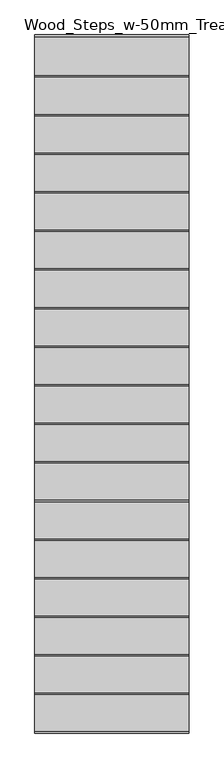
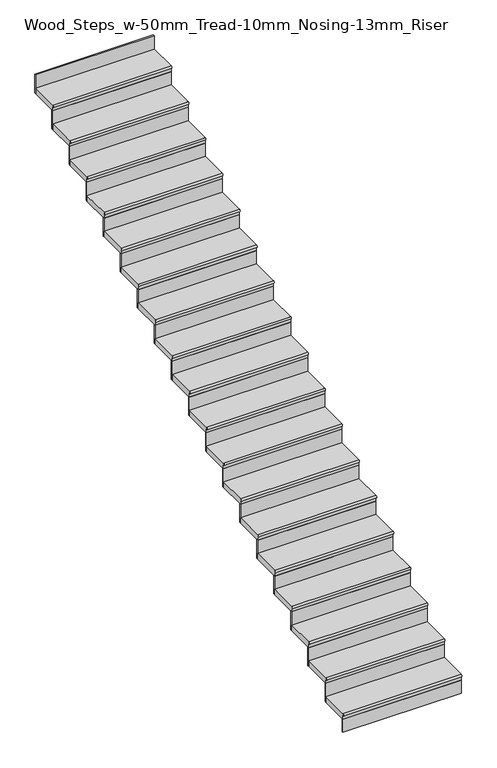
"""IFC4 building model written with IfcOpenShell, lengths in millimetres: stair flight geometry, Wood_Steps_w-50mm_Tread-10mm_Nosing-13mm_Riser."""

from ifc_helpers import new_model, si_unit, point, frame, frame_2d, origin, origin_with_axes, place, context, project, spatial, polyline, circle_curve, trimmed, segment, composite_curve, outline, extrude, source, transform, mapped, element, save


def wood_steps_w_50mm_tread_10mm_nosing_13mm_riser_22d6e456(model_context):
    return source(origin(), model_context, "Body", "SweptSolid", [
        extrude(outline(composite_curve([segment(polyline([(10202.4990528, 168.4210526), (10452.4990528, 168.4210526), (10452.4990528, 118.4210526), (10202.4990528, 118.4210526), (10202.4990528, 148.4210526)]), True, "CONTINUOUS"), segment(trimmed(circle_curve(frame_2d((10202.4990528, 158.4210526)), 10.0), [point((10202.4990528, 148.4210526))], [point((10202.4990528, 168.4210526))], False, "CARTESIAN"), True, "CONTINUOUS")], self_intersect=False)), frame((-6660.2000057, 0.0, 0.0), z_axis=(1.0, 0.0, 0.0), x_axis=(0.0, 1.0, 0.0)), (0.0, 0.0, 1.0), 1000.0),
        extrude(outline(polyline([(-5660.2000057, 10214.9990528), (-5660.2000057, 10202.4990528), (-6660.2000057, 10202.4990528), (-6660.2000057, 10214.9990528), (-5660.2000057, 10214.9990528)])), origin_with_axes(), (0.0, 0.0, 1.0), 118.4210526),
        extrude(outline(polyline([(-5660.2000057, 10464.9990528), (-5660.2000057, 10452.4990528), (-6660.2000057, 10452.4990528), (-6660.2000057, 10464.9990528), (-5660.2000057, 10464.9990528)])), frame((0.0, 0.0, 118.4210526), z_axis=(0.0, 0.0, 1.0), x_axis=(1.0, 0.0, 0.0)), (0.0, 0.0, 1.0), 168.4210526),
        extrude(outline(composite_curve([segment(polyline([(10452.4990528, 336.8421053), (10702.4990528, 336.8421053), (10702.4990528, 286.8421053), (10452.4990528, 286.8421053), (10452.4990528, 316.8421053)]), True, "CONTINUOUS"), segment(trimmed(circle_curve(frame_2d((10452.4990528, 326.8421053)), 10.0), [point((10452.4990528, 316.8421053))], [point((10452.4990528, 336.8421053))], False, "CARTESIAN"), True, "CONTINUOUS")], self_intersect=False)), frame((-6660.2000057, 0.0, 0.0), z_axis=(1.0, 0.0, 0.0), x_axis=(0.0, 1.0, 0.0)), (0.0, 0.0, 1.0), 1000.0),
        extrude(outline(polyline([(-5660.2000057, 10714.9990528), (-5660.2000057, 10702.4990528), (-6660.2000057, 10702.4990528), (-6660.2000057, 10714.9990528), (-5660.2000057, 10714.9990528)])), frame((0.0, 0.0, 286.8421053), z_axis=(0.0, 0.0, 1.0), x_axis=(1.0, 0.0, 0.0)), (0.0, 0.0, 1.0), 168.4210526),
        extrude(outline(composite_curve([segment(polyline([(10702.4990528, 505.2631579), (10952.4990528, 505.2631579), (10952.4990528, 455.2631579), (10702.4990528, 455.2631579), (10702.4990528, 485.2631579)]), True, "CONTINUOUS"), segment(trimmed(circle_curve(frame_2d((10702.4990528, 495.2631579)), 10.0), [point((10702.4990528, 485.2631579))], [point((10702.4990528, 505.2631579))], False, "CARTESIAN"), True, "CONTINUOUS")], self_intersect=False)), frame((-6660.2000057, 0.0, 0.0), z_axis=(1.0, 0.0, 0.0), x_axis=(0.0, 1.0, 0.0)), (0.0, 0.0, 1.0), 1000.0),
        extrude(outline(polyline([(-5660.2000057, 10964.9990528), (-5660.2000057, 10952.4990528), (-6660.2000057, 10952.4990528), (-6660.2000057, 10964.9990528), (-5660.2000057, 10964.9990528)])), frame((0.0, 0.0, 455.2631579), z_axis=(0.0, 0.0, 1.0), x_axis=(1.0, 0.0, 0.0)), (0.0, 0.0, 1.0), 168.4210526),
        extrude(outline(composite_curve([segment(polyline([(10952.4990528, 673.6842105), (11202.4990528, 673.6842105), (11202.4990528, 623.6842105), (10952.4990528, 623.6842105), (10952.4990528, 653.6842105)]), True, "CONTINUOUS"), segment(trimmed(circle_curve(frame_2d((10952.4990528, 663.6842105)), 10.0), [point((10952.4990528, 653.6842105))], [point((10952.4990528, 673.6842105))], False, "CARTESIAN"), True, "CONTINUOUS")], self_intersect=False)), frame((-6660.2000057, 0.0, 0.0), z_axis=(1.0, 0.0, 0.0), x_axis=(0.0, 1.0, 0.0)), (0.0, 0.0, 1.0), 1000.0),
        extrude(outline(polyline([(-5660.2000057, 11214.9990528), (-5660.2000057, 11202.4990528), (-6660.2000057, 11202.4990528), (-6660.2000057, 11214.9990528), (-5660.2000057, 11214.9990528)])), frame((0.0, 0.0, 623.6842105), z_axis=(0.0, 0.0, 1.0), x_axis=(1.0, 0.0, 0.0)), (0.0, 0.0, 1.0), 168.4210526),
        extrude(outline(composite_curve([segment(polyline([(11202.4990528, 842.1052632), (11452.4990528, 842.1052632), (11452.4990528, 792.1052632), (11202.4990528, 792.1052632), (11202.4990528, 822.1052632)]), True, "CONTINUOUS"), segment(trimmed(circle_curve(frame_2d((11202.4990528, 832.1052632)), 10.0), [point((11202.4990528, 822.1052632))], [point((11202.4990528, 842.1052632))], False, "CARTESIAN"), True, "CONTINUOUS")], self_intersect=False)), frame((-6660.2000057, 0.0, 0.0), z_axis=(1.0, 0.0, 0.0), x_axis=(0.0, 1.0, 0.0)), (0.0, 0.0, 1.0), 1000.0),
        extrude(outline(polyline([(-5660.2000057, 11464.9990528), (-5660.2000057, 11452.4990528), (-6660.2000057, 11452.4990528), (-6660.2000057, 11464.9990528), (-5660.2000057, 11464.9990528)])), frame((0.0, 0.0, 792.1052632), z_axis=(0.0, 0.0, 1.0), x_axis=(1.0, 0.0, 0.0)), (0.0, 0.0, 1.0), 168.4210526),
        extrude(outline(composite_curve([segment(polyline([(11452.4990528, 1010.5263158), (11702.4990528, 1010.5263158), (11702.4990528, 960.5263158), (11452.4990528, 960.5263158), (11452.4990528, 990.5263158)]), True, "CONTINUOUS"), segment(trimmed(circle_curve(frame_2d((11452.4990528, 1000.5263158)), 10.0), [point((11452.4990528, 990.5263158))], [point((11452.4990528, 1010.5263158))], False, "CARTESIAN"), True, "CONTINUOUS")], self_intersect=False)), frame((-6660.2000057, 0.0, 0.0), z_axis=(1.0, 0.0, 0.0), x_axis=(0.0, 1.0, 0.0)), (0.0, 0.0, 1.0), 1000.0),
        extrude(outline(polyline([(-5660.2000057, 11714.9990528), (-5660.2000057, 11702.4990528), (-6660.2000057, 11702.4990528), (-6660.2000057, 11714.9990528), (-5660.2000057, 11714.9990528)])), frame((0.0, 0.0, 960.5263158), z_axis=(0.0, 0.0, 1.0), x_axis=(1.0, 0.0, 0.0)), (0.0, 0.0, 1.0), 168.4210526),
        extrude(outline(composite_curve([segment(polyline([(11702.4990528, 1178.9473684), (11952.4990528, 1178.9473684), (11952.4990528, 1128.9473684), (11702.4990528, 1128.9473684), (11702.4990528, 1158.9473684)]), True, "CONTINUOUS"), segment(trimmed(circle_curve(frame_2d((11702.4990528, 1168.9473684)), 10.0), [point((11702.4990528, 1158.9473684))], [point((11702.4990528, 1178.9473684))], False, "CARTESIAN"), True, "CONTINUOUS")], self_intersect=False)), frame((-6660.2000057, 0.0, 0.0), z_axis=(1.0, 0.0, 0.0), x_axis=(0.0, 1.0, 0.0)), (0.0, 0.0, 1.0), 1000.0),
        extrude(outline(polyline([(-5660.2000057, 11964.9990528), (-5660.2000057, 11952.4990528), (-6660.2000057, 11952.4990528), (-6660.2000057, 11964.9990528), (-5660.2000057, 11964.9990528)])), frame((0.0, 0.0, 1128.9473684), z_axis=(0.0, 0.0, 1.0), x_axis=(1.0, 0.0, 0.0)), (0.0, 0.0, 1.0), 168.4210526),
        extrude(outline(composite_curve([segment(polyline([(11952.4990528, 1347.3684211), (12202.4990528, 1347.3684211), (12202.4990528, 1297.3684211), (11952.4990528, 1297.3684211), (11952.4990528, 1327.3684211)]), True, "CONTINUOUS"), segment(trimmed(circle_curve(frame_2d((11952.4990528, 1337.3684211)), 10.0), [point((11952.4990528, 1327.3684211))], [point((11952.4990528, 1347.3684211))], False, "CARTESIAN"), True, "CONTINUOUS")], self_intersect=False)), frame((-6660.2000057, 0.0, 0.0), z_axis=(1.0, 0.0, 0.0), x_axis=(0.0, 1.0, 0.0)), (0.0, 0.0, 1.0), 1000.0),
        extrude(outline(polyline([(-5660.2000057, 12214.9990528), (-5660.2000057, 12202.4990528), (-6660.2000057, 12202.4990528), (-6660.2000057, 12214.9990528), (-5660.2000057, 12214.9990528)])), frame((0.0, 0.0, 1297.3684211), z_axis=(0.0, 0.0, 1.0), x_axis=(1.0, 0.0, 0.0)), (0.0, 0.0, 1.0), 168.4210526),
        extrude(outline(composite_curve([segment(polyline([(12202.4990528, 1515.7894737), (12452.4990528, 1515.7894737), (12452.4990528, 1465.7894737), (12202.4990528, 1465.7894737), (12202.4990528, 1495.7894737)]), True, "CONTINUOUS"), segment(trimmed(circle_curve(frame_2d((12202.4990528, 1505.7894737)), 10.0), [point((12202.4990528, 1495.7894737))], [point((12202.4990528, 1515.7894737))], False, "CARTESIAN"), True, "CONTINUOUS")], self_intersect=False)), frame((-6660.2000057, 0.0, 0.0), z_axis=(1.0, 0.0, 0.0), x_axis=(0.0, 1.0, 0.0)), (0.0, 0.0, 1.0), 1000.0),
        extrude(outline(polyline([(-5660.2000057, 12464.9990528), (-5660.2000057, 12452.4990528), (-6660.2000057, 12452.4990528), (-6660.2000057, 12464.9990528), (-5660.2000057, 12464.9990528)])), frame((0.0, 0.0, 1465.7894737), z_axis=(0.0, 0.0, 1.0), x_axis=(1.0, 0.0, 0.0)), (0.0, 0.0, 1.0), 168.4210526),
        extrude(outline(composite_curve([segment(polyline([(12452.4990528, 1684.2105263), (12702.4990528, 1684.2105263), (12702.4990528, 1634.2105263), (12452.4990528, 1634.2105263), (12452.4990528, 1664.2105263)]), True, "CONTINUOUS"), segment(trimmed(circle_curve(frame_2d((12452.4990528, 1674.2105263)), 10.0), [point((12452.4990528, 1664.2105263))], [point((12452.4990528, 1684.2105263))], False, "CARTESIAN"), True, "CONTINUOUS")], self_intersect=False)), frame((-6660.2000057, 0.0, 0.0), z_axis=(1.0, 0.0, 0.0), x_axis=(0.0, 1.0, 0.0)), (0.0, 0.0, 1.0), 1000.0),
        extrude(outline(polyline([(-5660.2000057, 12714.9990528), (-5660.2000057, 12702.4990528), (-6660.2000057, 12702.4990528), (-6660.2000057, 12714.9990528), (-5660.2000057, 12714.9990528)])), frame((0.0, 0.0, 1634.2105263), z_axis=(0.0, 0.0, 1.0), x_axis=(1.0, 0.0, 0.0)), (0.0, 0.0, 1.0), 168.4210526),
        extrude(outline(composite_curve([segment(polyline([(12702.4990528, 1852.6315789), (12952.4990528, 1852.6315789), (12952.4990528, 1802.6315789), (12702.4990528, 1802.6315789), (12702.4990528, 1832.6315789)]), True, "CONTINUOUS"), segment(trimmed(circle_curve(frame_2d((12702.4990528, 1842.6315789)), 10.0), [point((12702.4990528, 1832.6315789))], [point((12702.4990528, 1852.6315789))], False, "CARTESIAN"), True, "CONTINUOUS")], self_intersect=False)), frame((-6660.2000057, 0.0, 0.0), z_axis=(1.0, 0.0, 0.0), x_axis=(0.0, 1.0, 0.0)), (0.0, 0.0, 1.0), 1000.0),
        extrude(outline(polyline([(-5660.2000057, 12964.9990528), (-5660.2000057, 12952.4990528), (-6660.2000057, 12952.4990528), (-6660.2000057, 12964.9990528), (-5660.2000057, 12964.9990528)])), frame((0.0, 0.0, 1802.6315789), z_axis=(0.0, 0.0, 1.0), x_axis=(1.0, 0.0, 0.0)), (0.0, 0.0, 1.0), 168.4210526),
        extrude(outline(composite_curve([segment(polyline([(12952.4990528, 2021.0526316), (13202.4990528, 2021.0526316), (13202.4990528, 1971.0526316), (12952.4990528, 1971.0526316), (12952.4990528, 2001.0526316)]), True, "CONTINUOUS"), segment(trimmed(circle_curve(frame_2d((12952.4990528, 2011.0526316)), 10.0), [point((12952.4990528, 2001.0526316))], [point((12952.4990528, 2021.0526316))], False, "CARTESIAN"), True, "CONTINUOUS")], self_intersect=False)), frame((-6660.2000057, 0.0, 0.0), z_axis=(1.0, 0.0, 0.0), x_axis=(0.0, 1.0, 0.0)), (0.0, 0.0, 1.0), 1000.0),
        extrude(outline(polyline([(-5660.2000057, 13214.9990528), (-5660.2000057, 13202.4990528), (-6660.2000057, 13202.4990528), (-6660.2000057, 13214.9990528), (-5660.2000057, 13214.9990528)])), frame((0.0, 0.0, 1971.0526316), z_axis=(0.0, 0.0, 1.0), x_axis=(1.0, 0.0, 0.0)), (0.0, 0.0, 1.0), 168.4210526),
        extrude(outline(composite_curve([segment(polyline([(13202.4990528, 2189.4736842), (13452.4990528, 2189.4736842), (13452.4990528, 2139.4736842), (13202.4990528, 2139.4736842), (13202.4990528, 2169.4736842)]), True, "CONTINUOUS"), segment(trimmed(circle_curve(frame_2d((13202.4990528, 2179.4736842)), 10.0), [point((13202.4990528, 2169.4736842))], [point((13202.4990528, 2189.4736842))], False, "CARTESIAN"), True, "CONTINUOUS")], self_intersect=False)), frame((-6660.2000057, 0.0, 0.0), z_axis=(1.0, 0.0, 0.0), x_axis=(0.0, 1.0, 0.0)), (0.0, 0.0, 1.0), 1000.0),
        extrude(outline(polyline([(-5660.2000057, 13464.9990528), (-5660.2000057, 13452.4990528), (-6660.2000057, 13452.4990528), (-6660.2000057, 13464.9990528), (-5660.2000057, 13464.9990528)])), frame((0.0, 0.0, 2139.4736842), z_axis=(0.0, 0.0, 1.0), x_axis=(1.0, 0.0, 0.0)), (0.0, 0.0, 1.0), 168.4210526),
        extrude(outline(composite_curve([segment(polyline([(13452.4990528, 2357.8947368), (13702.4990528, 2357.8947368), (13702.4990528, 2307.8947368), (13452.4990528, 2307.8947368), (13452.4990528, 2337.8947368)]), True, "CONTINUOUS"), segment(trimmed(circle_curve(frame_2d((13452.4990528, 2347.8947368)), 10.0), [point((13452.4990528, 2337.8947368))], [point((13452.4990528, 2357.8947368))], False, "CARTESIAN"), True, "CONTINUOUS")], self_intersect=False)), frame((-6660.2000057, 0.0, 0.0), z_axis=(1.0, 0.0, 0.0), x_axis=(0.0, 1.0, 0.0)), (0.0, 0.0, 1.0), 1000.0),
        extrude(outline(polyline([(-5660.2000057, 13714.9990528), (-5660.2000057, 13702.4990528), (-6660.2000057, 13702.4990528), (-6660.2000057, 13714.9990528), (-5660.2000057, 13714.9990528)])), frame((0.0, 0.0, 2307.8947368), z_axis=(0.0, 0.0, 1.0), x_axis=(1.0, 0.0, 0.0)), (0.0, 0.0, 1.0), 168.4210526),
        extrude(outline(composite_curve([segment(polyline([(13702.4990528, 2526.3157895), (13952.4990528, 2526.3157895), (13952.4990528, 2476.3157895), (13702.4990528, 2476.3157895), (13702.4990528, 2506.3157895)]), True, "CONTINUOUS"), segment(trimmed(circle_curve(frame_2d((13702.4990528, 2516.3157895)), 10.0), [point((13702.4990528, 2506.3157895))], [point((13702.4990528, 2526.3157895))], False, "CARTESIAN"), True, "CONTINUOUS")], self_intersect=False)), frame((-6660.2000057, 0.0, 0.0), z_axis=(1.0, 0.0, 0.0), x_axis=(0.0, 1.0, 0.0)), (0.0, 0.0, 1.0), 1000.0),
        extrude(outline(polyline([(-5660.2000057, 13964.9990528), (-5660.2000057, 13952.4990528), (-6660.2000057, 13952.4990528), (-6660.2000057, 13964.9990528), (-5660.2000057, 13964.9990528)])), frame((0.0, 0.0, 2476.3157895), z_axis=(0.0, 0.0, 1.0), x_axis=(1.0, 0.0, 0.0)), (0.0, 0.0, 1.0), 168.4210526),
        extrude(outline(composite_curve([segment(polyline([(13952.4990528, 2694.7368421), (14202.4990528, 2694.7368421), (14202.4990528, 2644.7368421), (13952.4990528, 2644.7368421), (13952.4990528, 2674.7368421)]), True, "CONTINUOUS"), segment(trimmed(circle_curve(frame_2d((13952.4990528, 2684.7368421)), 10.0), [point((13952.4990528, 2674.7368421))], [point((13952.4990528, 2694.7368421))], False, "CARTESIAN"), True, "CONTINUOUS")], self_intersect=False)), frame((-6660.2000057, 0.0, 0.0), z_axis=(1.0, 0.0, 0.0), x_axis=(0.0, 1.0, 0.0)), (0.0, 0.0, 1.0), 1000.0),
        extrude(outline(polyline([(-5660.2000057, 14214.9990528), (-5660.2000057, 14202.4990528), (-6660.2000057, 14202.4990528), (-6660.2000057, 14214.9990528), (-5660.2000057, 14214.9990528)])), frame((0.0, 0.0, 2644.7368421), z_axis=(0.0, 0.0, 1.0), x_axis=(1.0, 0.0, 0.0)), (0.0, 0.0, 1.0), 168.4210526),
        extrude(outline(composite_curve([segment(polyline([(14202.4990528, 2863.1578947), (14452.4990528, 2863.1578947), (14452.4990528, 2813.1578947), (14202.4990528, 2813.1578947), (14202.4990528, 2843.1578947)]), True, "CONTINUOUS"), segment(trimmed(circle_curve(frame_2d((14202.4990528, 2853.1578947)), 10.0), [point((14202.4990528, 2843.1578947))], [point((14202.4990528, 2863.1578947))], False, "CARTESIAN"), True, "CONTINUOUS")], self_intersect=False)), frame((-6660.2000057, 0.0, 0.0), z_axis=(1.0, 0.0, 0.0), x_axis=(0.0, 1.0, 0.0)), (0.0, 0.0, 1.0), 1000.0),
        extrude(outline(polyline([(-5660.2000057, 14464.9990528), (-5660.2000057, 14452.4990528), (-6660.2000057, 14452.4990528), (-6660.2000057, 14464.9990528), (-5660.2000057, 14464.9990528)])), frame((0.0, 0.0, 2813.1578947), z_axis=(0.0, 0.0, 1.0), x_axis=(1.0, 0.0, 0.0)), (0.0, 0.0, 1.0), 168.4210526),
        extrude(outline(polyline([(-5660.2000057, 14714.9990528), (-5660.2000057, 14702.4990528), (-6660.2000057, 14702.4990528), (-6660.2000057, 14714.9990528), (-5660.2000057, 14714.9990528)])), frame((0.0, 0.0, 2981.5789474), z_axis=(0.0, 0.0, 1.0), x_axis=(1.0, 0.0, 0.0)), (0.0, 0.0, 1.0), 168.4210526),
        extrude(outline(composite_curve([segment(polyline([(14452.4990528, 3031.5789474), (14702.4990528, 3031.5789474), (14702.4990528, 2981.5789474), (14452.4990528, 2981.5789474), (14452.4990528, 3011.5789474)]), True, "CONTINUOUS"), segment(trimmed(circle_curve(frame_2d((14452.4990528, 3021.5789474)), 10.0), [point((14452.4990528, 3011.5789474))], [point((14452.4990528, 3031.5789474))], False, "CARTESIAN"), True, "CONTINUOUS")], self_intersect=False)), frame((-6660.2000057, 0.0, 0.0), z_axis=(1.0, 0.0, 0.0), x_axis=(0.0, 1.0, 0.0)), (0.0, 0.0, 1.0), 1000.0),
    ])


if __name__ == "__main__":
    model = new_model("IFC4")
    model_context = context("Model", 3, world=origin())
    ifc_project = project(units=[si_unit("LENGTHUNIT", "METRE", prefix="MILLI")], contexts=[model_context])
    site = spatial("IfcSite", under=ifc_project)
    building = spatial("IfcBuilding", under=site)
    placement = place(None, origin())
    wood_steps_w_50mm_tread_10mm_nosing_13mm_riser_shape = wood_steps_w_50mm_tread_10mm_nosing_13mm_riser_22d6e456(model_context)
    element("IfcStairFlight", 1, ObjectType="Wood_Steps_w-50mm_Tread-10mm_Nosing-13mm_Riser", at=placement, inside=building, context=model_context, shape_type="MappedRepresentation", body=[
        mapped(wood_steps_w_50mm_tread_10mm_nosing_13mm_riser_shape, transform((0.0, 0.0, 0.0), x_axis=(1.0, 0.0, 0.0), y_axis=(0.0, 1.0, 0.0), z_axis=(0.0, 0.0, 1.0))),
    ])
    save(model, "model.ifc")

# Revit data of these elements
# Element 1 (IfcStairFlight, "Wood_Steps_w-50mm_Tread-10mm_Nosing-13mm_Riser")
#   Materials on its faces: "Oak Flooring"
# Materials
#   "Oak Flooring": class "Wood", colour RGB 212 179 113, transparency 0, Description = "Quercus Rubra", Cost = 0
